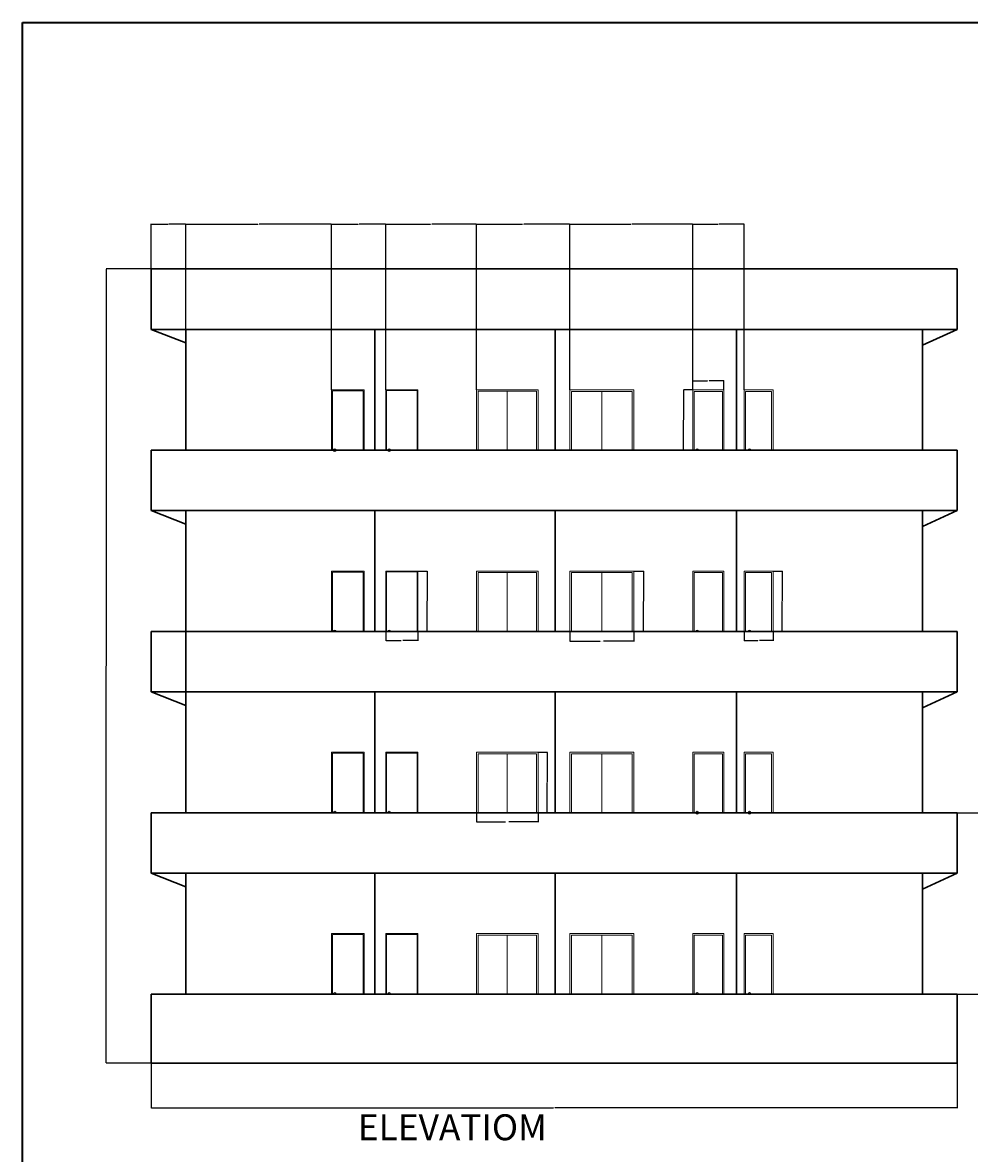
# Model space of a CAD drawing. Units: inches. Extents: x 1944 to 3454, y 1352 to 3055.
# Tile 16 of 17: x 1944 to 2602, y 2269 to 3055. Entities that reach past the tile are written whole.
import ezdxf

# ---------------------------------------------------------------- set-up
doc = ezdxf.new("R2010")
doc.units = ezdxf.units.IN
for name, color, linetype, lineweight in [('A-ANNO-DIMS', 2, 'Continuous', 18), ('A-ANNO-TITL', 7, 'Continuous', 30), ('A-ANNO-TTLB', 7, 'Continuous', 35), ('A-ELEV', 7, 'Continuous', 30), ('A-ELEV-DOOR', 3, 'Continuous', 18), ('A-ELEV-GLAZ', 4, 'Continuous', 18)]:
    doc.layers.add(name, color=color, linetype=linetype, lineweight=lineweight)
doc.styles.get("Standard").update_dxf_attribs({"font": 'arial.ttf'})
doc.dimstyles.get("Standard").update_dxf_attribs({"dimtxt": 0.18, "dimasz": 0.18, "dimexe": 0.18, "dimexo": 0.0625, "dimgap": 0.09, "dimtad": 0, "dimtih": 1, "dimtoh": 1, "dimdec": 4, "dimzin": 0, "dimdsep": 46, "dimtxsty": 'Standard', "dimcen": 0.09, "dimadec": 0, "dimazin": 0, "dimtfac": 1, "dimtdec": 4, "dimtofl": 0, "dimtmove": 0, "dimatfit": 3, "dimfxl": 1, "dimtolj": 1, "dimtzin": 0, "dimarcsym": 0})

# ---------------------------------------------------------------- blocks, each defined once
blk = doc.blocks.new('ELEV-DOOR-22.35IN-01')
for p, q in [((0, 42), (0, 0)), ((0, 42), (22.35, 42)), ((0, 42), (0, 0)), ((0, 42), (22.35, 42)), ((22.35, 42), (22.35, 0)), ((22.35, 42), (22.35, 0))]:
    blk.add_line(p, q)
blk.add_lwpolyline([(0.46, 0), (0.46, 41.46), (21.87, 41.46), (21.87, 0)])
blk.add_arc((2.34, 0), 0.993, 0, 180)
blk = doc.blocks.new('ELEV-DOOR-21.74IN-01')
for p, q in [((0, 42), (0, 0)), ((0, 42), (21.74, 42)), ((0, 42), (0, 0)), ((0, 42), (21.74, 42)), ((21.74, 42), (21.74, 0)), ((21.74, 42), (21.74, 0))]:
    blk.add_line(p, q)
blk.add_lwpolyline([(1.03, 0), (1.03, 40.92), (20.81, 40.92), (20.81, 0)])
blk.add_arc((3.12, 0), 0.993, 0, 180)
blk = doc.blocks.new('ELEV-DOOR-20.24IN-01')
for p, q in [((0, 42), (0, 0)), ((0, 42), (20.24, 42)), ((0, 42), (0, 0)), ((0, 42), (20.24, 42)), ((20.24, 42), (20.24, 0)), ((20.24, 42), (20.24, 0))]:
    blk.add_line(p, q)
blk.add_lwpolyline([(1.07, 0), (1.07, 40.9), (18.98, 40.9), (18.98, 0)])
blk.add_arc((3.81, 0), 0.993, 0, 180)
blk = doc.blocks.new('ELEV-GLAZ-42.86IN-01')
for p, q in [((0, 42), (0, 0)), ((0, 42), (42.86, 42)), ((0, 42), (0, 0)), ((0, 42), (42.86, 42)), ((21.49, 41), (21.49, 0)), ((42.86, 42), (42.86, 0)), ((42.86, 42), (42.86, 0))]:
    blk.add_line(p, q)
blk.add_lwpolyline([(1.15, 0), (1.15, 41), (41.83, 41), (41.83, 0)])
blk = doc.blocks.new('ELEV-GLAZ-44.51IN-01')
for p, q in [((0, 42), (0, 0)), ((0, 42), (44.51, 42)), ((0, 42), (0, 0)), ((0, 42), (44.51, 42)), ((22.21, 40.89), (22.21, 0)), ((44.51, 42), (44.51, 0)), ((44.51, 42), (44.51, 0))]:
    blk.add_line(p, q)
blk.add_lwpolyline([(1.11, 0), (1.11, 40.89), (43.32, 40.89), (43.32, 0)])
blk = doc.blocks.new('*D162')
at = {"layer": 'A-ANNO-DIMS', "color": 0, "lineweight": -2, "transparency": 16777216}
for p, q in [((2259.53, 2505.32), (2259.53, 2498.78)), ((2302.38, 2505.32), (2302.38, 2498.78)), ((2259.71, 2498.96), (2279.84, 2498.96)), ((2302.2, 2498.96), (2282.07, 2498.96))]:
    blk.add_line(p, q, dxfattribs=at)
at = {"layer": 'A-ANNO-DIMS', "color": 0, "transparency": 16777216}
for points in [[(2259.71, 2498.99), (2259.71, 2498.93), (2259.53, 2498.96)], [(2302.2, 2498.99), (2302.2, 2498.93), (2302.38, 2498.96)]]:
    blk.add_solid(points, dxfattribs=at)
at = {"layer": 'Defpoints', "color": 0, "transparency": 16777216}
for p in [(2259.53, 2505.38), (2302.38, 2505.38), (2302.38, 2498.96)]:
    blk.add_point(p, dxfattribs=at)
at = {"layer": 'A-ANNO-DIMS', "color": 0, "transparency": 16777216, "insert": (2280.96, 2498.96), "char_height": 0.18, "attachment_point": 5}
blk.add_mtext('\\A1;GLAZING 43 TYP.', dxfattribs=at)
blk = doc.blocks.new('*D163')
at = {"layer": 'A-ANNO-DIMS', "color": 0, "lineweight": -2, "transparency": 16777216}
for p, q in [((2302.45, 2547.38), (2308.99, 2547.38)), ((2308.81, 2547.2), (2308.81, 2526.56)), ((2308.81, 2505.56), (2308.81, 2526.2)), ((2302.45, 2505.38), (2308.99, 2505.38))]:
    blk.add_line(p, q, dxfattribs=at)
at = {"layer": 'A-ANNO-DIMS', "color": 0, "transparency": 16777216}
for points in [[(2308.78, 2547.2), (2308.84, 2547.2), (2308.81, 2547.38)], [(2308.78, 2505.56), (2308.84, 2505.56), (2308.81, 2505.38)]]:
    blk.add_solid(points, dxfattribs=at)
at = {"layer": 'Defpoints', "color": 0, "transparency": 16777216}
for p in [(2302.38, 2547.38), (2308.81, 2547.38), (2302.38, 2505.38)]:
    blk.add_point(p, dxfattribs=at)
at = {"layer": 'A-ANNO-DIMS', "color": 0, "transparency": 16777216, "insert": (2308.81, 2526.38), "char_height": 0.18, "attachment_point": 5}
blk.add_mtext('\\A1;42 TYP.', dxfattribs=at)
blk = doc.blocks.new('*D164')
at = {"layer": 'A-ANNO-DIMS', "color": 0, "lineweight": -2, "transparency": 16777216}
for p, q in [((2324.52, 2631.32), (2324.52, 2624.53)), ((2369.03, 2631.32), (2369.03, 2624.53)), ((2324.7, 2624.71), (2345.66, 2624.71)), ((2368.85, 2624.71), (2347.89, 2624.71))]:
    blk.add_line(p, q, dxfattribs=at)
at = {"layer": 'A-ANNO-DIMS', "color": 0, "transparency": 16777216}
for points in [[(2324.7, 2624.74), (2324.7, 2624.68), (2324.52, 2624.71)], [(2368.85, 2624.74), (2368.85, 2624.68), (2369.03, 2624.71)]]:
    blk.add_solid(points, dxfattribs=at)
at = {"layer": 'Defpoints', "color": 0, "transparency": 16777216}
for p in [(2324.52, 2631.38), (2369.03, 2631.38), (2369.03, 2624.71)]:
    blk.add_point(p, dxfattribs=at)
at = {"layer": 'A-ANNO-DIMS', "color": 0, "transparency": 16777216, "insert": (2346.78, 2624.71), "char_height": 0.18, "attachment_point": 5}
blk.add_mtext('\\A1;GLAZING 45 TYP.', dxfattribs=at)
blk = doc.blocks.new('*D165')
at = {"layer": 'A-ANNO-DIMS', "color": 0, "lineweight": -2, "transparency": 16777216}
for p, q in [((2369.1, 2673.38), (2375.89, 2673.38)), ((2375.71, 2673.2), (2375.71, 2652.56)), ((2375.71, 2631.56), (2375.71, 2652.2)), ((2369.1, 2631.38), (2375.89, 2631.38))]:
    blk.add_line(p, q, dxfattribs=at)
at = {"layer": 'A-ANNO-DIMS', "color": 0, "transparency": 16777216}
for points in [[(2375.68, 2673.2), (2375.74, 2673.2), (2375.71, 2673.38)], [(2375.68, 2631.56), (2375.74, 2631.56), (2375.71, 2631.38)]]:
    blk.add_solid(points, dxfattribs=at)
at = {"layer": 'Defpoints', "color": 0, "transparency": 16777216}
for p in [(2369.03, 2673.38), (2375.71, 2673.38), (2369.03, 2631.38)]:
    blk.add_point(p, dxfattribs=at)
at = {"layer": 'A-ANNO-DIMS', "color": 0, "transparency": 16777216, "insert": (2375.71, 2652.38), "char_height": 0.18, "attachment_point": 5}
blk.add_mtext('\\A1;42 TYP.', dxfattribs=at)
blk = doc.blocks.new('*D166')
at = {"layer": 'A-ANNO-DIMS', "color": 0, "lineweight": -2, "transparency": 16777216}
for p, q in [((2218.95, 2673.38), (2225.37, 2673.38)), ((2225.19, 2673.2), (2225.19, 2652.57)), ((2225.19, 2631.56), (2225.19, 2652.2)), ((2218.95, 2631.38), (2225.37, 2631.38))]:
    blk.add_line(p, q, dxfattribs=at)
at = {"layer": 'A-ANNO-DIMS', "color": 0, "transparency": 16777216}
for points in [[(2225.16, 2673.2), (2225.22, 2673.2), (2225.19, 2673.38)], [(2225.16, 2631.56), (2225.22, 2631.56), (2225.19, 2631.38)]]:
    blk.add_solid(points, dxfattribs=at)
at = {"layer": 'Defpoints', "color": 0, "transparency": 16777216}
for p in [(2218.89, 2673.38), (2225.19, 2673.38), (2218.89, 2631.38)]:
    blk.add_point(p, dxfattribs=at)
at = {"layer": 'A-ANNO-DIMS', "color": 0, "transparency": 16777216, "insert": (2225.19, 2652.38), "char_height": 0.18, "attachment_point": 5}
blk.add_mtext('\\A1;DOOR 42 TYP.', dxfattribs=at)
blk = doc.blocks.new('*D167')
at = {"layer": 'A-ANNO-DIMS', "color": 0, "lineweight": -2, "transparency": 16777216}
for p, q in [((2196.54, 2631.32), (2196.54, 2624.9)), ((2218.89, 2631.32), (2218.89, 2624.9)), ((2196.72, 2625.08), (2207.18, 2625.08)), ((2218.71, 2625.08), (2208.24, 2625.08))]:
    blk.add_line(p, q, dxfattribs=at)
at = {"layer": 'A-ANNO-DIMS', "color": 0, "transparency": 16777216}
for points in [[(2196.72, 2625.11), (2196.72, 2625.05), (2196.54, 2625.08)], [(2218.71, 2625.11), (2218.71, 2625.05), (2218.89, 2625.08)]]:
    blk.add_solid(points, dxfattribs=at)
at = {"layer": 'Defpoints', "color": 0, "transparency": 16777216}
for p in [(2196.54, 2631.38), (2218.89, 2631.38), (2218.89, 2625.08)]:
    blk.add_point(p, dxfattribs=at)
at = {"layer": 'A-ANNO-DIMS', "color": 0, "transparency": 16777216, "insert": (2207.71, 2625.08), "char_height": 0.18, "attachment_point": 5}
blk.add_mtext('\\A1;22 TYP.', dxfattribs=at)
blk = doc.blocks.new('*D168')
at = {"layer": 'A-ANNO-DIMS', "color": 0, "lineweight": -2, "transparency": 16777216}
for p, q in [((2409.85, 2799.38), (2403.43, 2799.38)), ((2403.61, 2799.2), (2403.61, 2778.57)), ((2403.61, 2757.56), (2403.61, 2778.2)), ((2409.85, 2757.38), (2403.43, 2757.38))]:
    blk.add_line(p, q, dxfattribs=at)
at = {"layer": 'A-ANNO-DIMS', "color": 0, "transparency": 16777216}
for points in [[(2403.58, 2799.2), (2403.64, 2799.2), (2403.61, 2799.38)], [(2403.58, 2757.56), (2403.64, 2757.56), (2403.61, 2757.38)]]:
    blk.add_solid(points, dxfattribs=at)
at = {"layer": 'Defpoints', "color": 0, "transparency": 16777216}
for p in [(2403.61, 2799.38), (2409.91, 2799.38), (2409.91, 2757.38)]:
    blk.add_point(p, dxfattribs=at)
at = {"layer": 'A-ANNO-DIMS', "color": 0, "transparency": 16777216, "insert": (2403.61, 2778.38), "char_height": 0.18, "attachment_point": 5}
blk.add_mtext('\\A1;DOOR 42 TYP.', dxfattribs=at)
blk = doc.blocks.new('*D169')
at = {"layer": 'A-ANNO-DIMS', "color": 0, "lineweight": -2, "transparency": 16777216}
for p, q in [((2409.91, 2799.45), (2409.91, 2805.86)), ((2410.09, 2805.68), (2420.26, 2805.68)), ((2431.48, 2805.68), (2421.31, 2805.68)), ((2431.66, 2799.45), (2431.66, 2805.86))]:
    blk.add_line(p, q, dxfattribs=at)
at = {"layer": 'A-ANNO-DIMS', "color": 0, "transparency": 16777216}
for points in [[(2410.09, 2805.71), (2410.09, 2805.65), (2409.91, 2805.68)], [(2431.48, 2805.71), (2431.48, 2805.65), (2431.66, 2805.68)]]:
    blk.add_solid(points, dxfattribs=at)
at = {"layer": 'Defpoints', "color": 0, "transparency": 16777216}
for p in [(2409.91, 2799.38), (2431.66, 2805.68), (2431.66, 2799.38)]:
    blk.add_point(p, dxfattribs=at)
at = {"layer": 'A-ANNO-DIMS', "color": 0, "transparency": 16777216, "insert": (2420.79, 2805.68), "char_height": 0.18, "attachment_point": 5}
blk.add_mtext('\\A1;22 TYP.', dxfattribs=at)
blk = doc.blocks.new('*D170')
at = {"layer": 'A-ANNO-DIMS', "color": 0, "lineweight": -2, "transparency": 16777216}
for p, q in [((2465.95, 2673.38), (2472.37, 2673.38)), ((2472.19, 2673.2), (2472.19, 2652.57)), ((2472.19, 2631.56), (2472.19, 2652.2)), ((2465.95, 2631.38), (2472.37, 2631.38))]:
    blk.add_line(p, q, dxfattribs=at)
at = {"layer": 'A-ANNO-DIMS', "color": 0, "transparency": 16777216}
for points in [[(2472.16, 2673.2), (2472.22, 2673.2), (2472.19, 2673.38)], [(2472.16, 2631.56), (2472.22, 2631.56), (2472.19, 2631.38)]]:
    blk.add_solid(points, dxfattribs=at)
at = {"layer": 'Defpoints', "color": 0, "transparency": 16777216}
for p in [(2465.89, 2673.38), (2472.19, 2673.38), (2465.89, 2631.38)]:
    blk.add_point(p, dxfattribs=at)
at = {"layer": 'A-ANNO-DIMS', "color": 0, "transparency": 16777216, "insert": (2472.19, 2652.38), "char_height": 0.18, "attachment_point": 5}
blk.add_mtext('\\A1;DOOR 42 TYP.', dxfattribs=at)
blk = doc.blocks.new('*D171')
at = {"layer": 'A-ANNO-DIMS', "color": 0, "lineweight": -2, "transparency": 16777216}
for p, q in [((2445.66, 2631.32), (2445.66, 2624.9)), ((2465.89, 2631.32), (2465.89, 2624.9)), ((2445.84, 2625.08), (2455.24, 2625.08)), ((2465.71, 2625.08), (2456.3, 2625.08))]:
    blk.add_line(p, q, dxfattribs=at)
at = {"layer": 'A-ANNO-DIMS', "color": 0, "transparency": 16777216}
for points in [[(2445.84, 2625.11), (2445.84, 2625.05), (2445.66, 2625.08)], [(2465.71, 2625.11), (2465.71, 2625.05), (2465.89, 2625.08)]]:
    blk.add_solid(points, dxfattribs=at)
at = {"layer": 'Defpoints', "color": 0, "transparency": 16777216}
for p in [(2445.66, 2631.38), (2465.89, 2631.38), (2465.89, 2625.08)]:
    blk.add_point(p, dxfattribs=at)
at = {"layer": 'A-ANNO-DIMS', "color": 0, "transparency": 16777216, "insert": (2455.77, 2625.08), "char_height": 0.18, "attachment_point": 5}
blk.add_mtext('\\A1;20 TYP.', dxfattribs=at)
blk = doc.blocks.new('*D199')
at = {"layer": 'A-ANNO-DIMS', "color": 0, "lineweight": -2, "transparency": 16777216}
for p, q in [((2033.32, 2331.32), (2033.32, 2300)), ((2593.82, 2331.32), (2593.82, 2300)), ((2033.5, 2300.18), (2313.18, 2300.18)), ((2593.64, 2300.18), (2313.97, 2300.18))]:
    blk.add_line(p, q, dxfattribs=at)
at = {"layer": 'A-ANNO-DIMS', "color": 0, "transparency": 16777216}
for points in [[(2033.5, 2300.21), (2033.5, 2300.15), (2033.32, 2300.18)], [(2593.64, 2300.21), (2593.64, 2300.15), (2593.82, 2300.18)]]:
    blk.add_solid(points, dxfattribs=at)
at = {"layer": 'Defpoints', "color": 0, "transparency": 16777216}
for p in [(2033.32, 2331.38), (2593.82, 2331.38), (2593.82, 2300.18)]:
    blk.add_point(p, dxfattribs=at)
at = {"layer": 'A-ANNO-DIMS', "color": 0, "transparency": 16777216, "insert": (2313.57, 2300.18), "char_height": 0.18, "attachment_point": 5}
blk.add_mtext('\\A1;560.5', dxfattribs=at)
blk = doc.blocks.new('*D200')
at = {"layer": 'A-ANNO-DIMS', "color": 0, "lineweight": -2, "transparency": 16777216}
for p, q in [((2033.26, 2883.38), (2001.94, 2883.38)), ((2002.12, 2883.2), (2002.12, 2607.57)), ((2002.12, 2331.56), (2002.12, 2607.2)), ((2033.26, 2331.38), (2001.94, 2331.38))]:
    blk.add_line(p, q, dxfattribs=at)
at = {"layer": 'A-ANNO-DIMS', "color": 0, "transparency": 16777216}
for points in [[(2002.09, 2883.2), (2002.15, 2883.2), (2002.12, 2883.38)], [(2002.09, 2331.56), (2002.15, 2331.56), (2002.12, 2331.38)]]:
    blk.add_solid(points, dxfattribs=at)
at = {"layer": 'Defpoints', "color": 0, "transparency": 16777216}
for p in [(2002.12, 2883.38), (2033.32, 2883.38), (2033.32, 2331.38)]:
    blk.add_point(p, dxfattribs=at)
at = {"layer": 'A-ANNO-DIMS', "color": 0, "transparency": 16777216, "insert": (2002.12, 2607.38), "char_height": 0.18, "attachment_point": 5}
blk.add_mtext('\\A1;552', dxfattribs=at)
blk = doc.blocks.new('*D201')
at = {"layer": 'A-ANNO-DIMS', "color": 0, "lineweight": -2, "transparency": 16777216}
for p, q in [((2593.88, 2505.38), (2625.2, 2505.38)), ((2625.02, 2505.2), (2625.02, 2442.57)), ((2625.02, 2379.56), (2625.02, 2442.2)), ((2593.88, 2379.38), (2625.2, 2379.38))]:
    blk.add_line(p, q, dxfattribs=at)
at = {"layer": 'A-ANNO-DIMS', "color": 0, "transparency": 16777216}
for points in [[(2624.99, 2505.2), (2625.05, 2505.2), (2625.02, 2505.38)], [(2624.99, 2379.56), (2625.05, 2379.56), (2625.02, 2379.38)]]:
    blk.add_solid(points, dxfattribs=at)
at = {"layer": 'Defpoints', "color": 0, "transparency": 16777216}
for p in [(2593.82, 2505.38), (2625.02, 2505.38), (2593.82, 2379.38)]:
    blk.add_point(p, dxfattribs=at)
at = {"layer": 'A-ANNO-DIMS', "color": 0, "transparency": 16777216, "insert": (2625.02, 2442.38), "char_height": 0.18, "attachment_point": 5}
blk.add_mtext('\\A1;126', dxfattribs=at)
blk = doc.blocks.new('*D202')
at = {"layer": 'A-ANNO-DIMS', "color": 0, "lineweight": -2, "transparency": 16777216}
for p, q in [((2033.32, 2841.45), (2033.32, 2914.76)), ((2033.5, 2914.58), (2045.1, 2914.58)), ((2057.14, 2914.58), (2045.54, 2914.58)), ((2057.32, 2841.45), (2057.32, 2914.76))]:
    blk.add_line(p, q, dxfattribs=at)
at = {"layer": 'A-ANNO-DIMS', "color": 0, "transparency": 16777216}
for points in [[(2033.5, 2914.61), (2033.5, 2914.55), (2033.32, 2914.58)], [(2057.14, 2914.61), (2057.14, 2914.55), (2057.32, 2914.58)]]:
    blk.add_solid(points, dxfattribs=at)
at = {"layer": 'Defpoints', "color": 0, "transparency": 16777216}
for p in [(2057.32, 2914.58), (2033.32, 2841.38), (2057.32, 2841.38)]:
    blk.add_point(p, dxfattribs=at)
at = {"layer": 'A-ANNO-DIMS', "color": 0, "transparency": 16777216, "insert": (2045.32, 2914.58), "char_height": 0.18, "attachment_point": 5}
blk.add_mtext('\\A1;24', dxfattribs=at)
blk = doc.blocks.new('*D203')
at = {"layer": 'A-ANNO-DIMS', "color": 0, "lineweight": -2, "transparency": 16777216}
for p, q in [((2057.32, 2841.45), (2057.32, 2914.76)), ((2057.5, 2914.58), (2107.56, 2914.58)), ((2158.52, 2914.58), (2108.47, 2914.58)), ((2158.7, 2799.45), (2158.7, 2914.76))]:
    blk.add_line(p, q, dxfattribs=at)
at = {"layer": 'A-ANNO-DIMS', "color": 0, "transparency": 16777216}
for points in [[(2057.5, 2914.61), (2057.5, 2914.55), (2057.32, 2914.58)], [(2158.52, 2914.61), (2158.52, 2914.55), (2158.7, 2914.58)]]:
    blk.add_solid(points, dxfattribs=at)
at = {"layer": 'Defpoints', "color": 0, "transparency": 16777216}
for p in [(2158.7, 2914.58), (2057.32, 2841.38), (2158.7, 2799.38)]:
    blk.add_point(p, dxfattribs=at)
at = {"layer": 'A-ANNO-DIMS', "color": 0, "transparency": 16777216, "insert": (2108.01, 2914.58), "char_height": 0.18, "attachment_point": 5}
blk.add_mtext('\\A1;101.38', dxfattribs=at)
blk = doc.blocks.new('*D204')
at = {"layer": 'A-ANNO-DIMS', "color": 0, "lineweight": -2, "transparency": 16777216}
for p, q in [((2158.7, 2799.45), (2158.7, 2914.76)), ((2158.88, 2914.58), (2177.23, 2914.58)), ((2196.36, 2914.58), (2178.01, 2914.58)), ((2196.54, 2799.45), (2196.54, 2914.76))]:
    blk.add_line(p, q, dxfattribs=at)
at = {"layer": 'A-ANNO-DIMS', "color": 0, "transparency": 16777216}
for points in [[(2158.88, 2914.61), (2158.88, 2914.55), (2158.7, 2914.58)], [(2196.36, 2914.61), (2196.36, 2914.55), (2196.54, 2914.58)]]:
    blk.add_solid(points, dxfattribs=at)
at = {"layer": 'Defpoints', "color": 0, "transparency": 16777216}
for p in [(2196.54, 2914.58), (2158.7, 2799.38), (2196.54, 2799.38)]:
    blk.add_point(p, dxfattribs=at)
at = {"layer": 'A-ANNO-DIMS', "color": 0, "transparency": 16777216, "insert": (2177.62, 2914.58), "char_height": 0.18, "attachment_point": 5}
blk.add_mtext('\\A1;37.84', dxfattribs=at)
blk = doc.blocks.new('*D205')
at = {"layer": 'A-ANNO-DIMS', "color": 0, "lineweight": -2, "transparency": 16777216}
for p, q in [((2196.54, 2799.45), (2196.54, 2914.76)), ((2196.72, 2914.58), (2227.64, 2914.58)), ((2259.35, 2914.58), (2228.43, 2914.58)), ((2259.53, 2799.45), (2259.53, 2914.76))]:
    blk.add_line(p, q, dxfattribs=at)
at = {"layer": 'A-ANNO-DIMS', "color": 0, "transparency": 16777216}
for points in [[(2196.72, 2914.61), (2196.72, 2914.55), (2196.54, 2914.58)], [(2259.35, 2914.61), (2259.35, 2914.55), (2259.53, 2914.58)]]:
    blk.add_solid(points, dxfattribs=at)
at = {"layer": 'Defpoints', "color": 0, "transparency": 16777216}
for p in [(2259.53, 2914.58), (2196.54, 2799.38), (2259.53, 2799.38)]:
    blk.add_point(p, dxfattribs=at)
at = {"layer": 'A-ANNO-DIMS', "color": 0, "transparency": 16777216, "insert": (2228.03, 2914.58), "char_height": 0.18, "attachment_point": 5}
blk.add_mtext('\\A1;62.99', dxfattribs=at)
blk = doc.blocks.new('*D206')
at = {"layer": 'A-ANNO-DIMS', "color": 0, "lineweight": -2, "transparency": 16777216}
for p, q in [((2259.53, 2799.45), (2259.53, 2914.76)), ((2259.71, 2914.58), (2291.63, 2914.58)), ((2324.34, 2914.58), (2292.42, 2914.58)), ((2324.52, 2799.45), (2324.52, 2914.76))]:
    blk.add_line(p, q, dxfattribs=at)
at = {"layer": 'A-ANNO-DIMS', "color": 0, "transparency": 16777216}
for points in [[(2259.71, 2914.61), (2259.71, 2914.55), (2259.53, 2914.58)], [(2324.34, 2914.61), (2324.34, 2914.55), (2324.52, 2914.58)]]:
    blk.add_solid(points, dxfattribs=at)
at = {"layer": 'Defpoints', "color": 0, "transparency": 16777216}
for p in [(2324.52, 2914.58), (2259.53, 2799.38), (2324.52, 2799.38)]:
    blk.add_point(p, dxfattribs=at)
at = {"layer": 'A-ANNO-DIMS', "color": 0, "transparency": 16777216, "insert": (2292.03, 2914.58), "char_height": 0.18, "attachment_point": 5}
blk.add_mtext('\\A1;64.99', dxfattribs=at)
blk = doc.blocks.new('*D207')
at = {"layer": 'A-ANNO-DIMS', "color": 0, "lineweight": -2, "transparency": 16777216}
for p, q in [((2324.52, 2799.45), (2324.52, 2914.76)), ((2324.7, 2914.58), (2366.89, 2914.58)), ((2409.73, 2914.58), (2367.54, 2914.58)), ((2409.91, 2799.45), (2409.91, 2914.76))]:
    blk.add_line(p, q, dxfattribs=at)
at = {"layer": 'A-ANNO-DIMS', "color": 0, "transparency": 16777216}
for points in [[(2324.7, 2914.61), (2324.7, 2914.55), (2324.52, 2914.58)], [(2409.73, 2914.61), (2409.73, 2914.55), (2409.91, 2914.58)]]:
    blk.add_solid(points, dxfattribs=at)
at = {"layer": 'Defpoints', "color": 0, "transparency": 16777216}
for p in [(2409.91, 2914.58), (2324.52, 2799.38), (2409.91, 2799.38)]:
    blk.add_point(p, dxfattribs=at)
at = {"layer": 'A-ANNO-DIMS', "color": 0, "transparency": 16777216, "insert": (2367.22, 2914.58), "char_height": 0.18, "attachment_point": 5}
blk.add_mtext('\\A1;85.4', dxfattribs=at)
blk = doc.blocks.new('*D208')
at = {"layer": 'A-ANNO-DIMS', "color": 0, "lineweight": -2, "transparency": 16777216}
for p, q in [((2409.91, 2799.45), (2409.91, 2914.76)), ((2410.09, 2914.58), (2427.39, 2914.58)), ((2445.48, 2914.58), (2428.18, 2914.58)), ((2445.66, 2799.45), (2445.66, 2914.76))]:
    blk.add_line(p, q, dxfattribs=at)
at = {"layer": 'A-ANNO-DIMS', "color": 0, "transparency": 16777216}
for points in [[(2410.09, 2914.61), (2410.09, 2914.55), (2409.91, 2914.58)], [(2445.48, 2914.61), (2445.48, 2914.55), (2445.66, 2914.58)]]:
    blk.add_solid(points, dxfattribs=at)
at = {"layer": 'Defpoints', "color": 0, "transparency": 16777216}
for p in [(2445.66, 2914.58), (2409.91, 2799.38), (2445.66, 2799.38)]:
    blk.add_point(p, dxfattribs=at)
at = {"layer": 'A-ANNO-DIMS', "color": 0, "transparency": 16777216, "insert": (2427.78, 2914.58), "char_height": 0.18, "attachment_point": 5}
blk.add_mtext('\\A1;35.74', dxfattribs=at)

msp = doc.modelspace()

# ---------------------------------------------------------------- linework, layer by layer
at = {"layer": 'A-ANNO-TTLB'}
msp.add_lwpolyline([(1943.914, 3054.605), (3453.633, 3054.605), (3453.633, 1351.76), (1943.914, 1351.76)], close=True, dxfattribs=at)
at = {"layer": 'A-ELEV'}
for p, q in [((2033.322, 2883.384), (2593.822, 2883.384)), ((2033.322, 2841.384), (2033.322, 2883.384)), ((2593.822, 2841.384), (2593.822, 2883.384)), ((2033.322, 2841.384), (2593.822, 2841.384)), ((2033.322, 2841.384), (2057.322, 2831.986)), ((2057.322, 2841.384), (2057.322, 2757.384)), ((2188.947, 2757.384), (2188.947, 2841.384)), ((2314.352, 2757.384), (2314.352, 2841.384)), ((2440.322, 2757.384), (2440.322, 2841.384)), ((2569.822, 2841.384), (2569.822, 2757.384)), ((2593.822, 2841.384), (2569.822, 2830.307)), ((2033.322, 2757.384), (2593.822, 2757.384)), ((2033.322, 2715.384), (2033.322, 2757.384)), ((2593.822, 2715.384), (2593.822, 2757.384)), ((2033.322, 2715.384), (2593.822, 2715.384)), ((2033.322, 2715.384), (2057.322, 2705.986)), ((2057.322, 2715.384), (2057.322, 2583.384)), ((2057.322, 2715.384), (2057.322, 2709.384)), ((2188.947, 2631.384), (2188.947, 2715.384)), ((2314.352, 2631.384), (2314.352, 2715.384)), ((2440.322, 2631.384), (2440.322, 2715.384)), ((2569.822, 2715.384), (2569.822, 2631.384)), ((2569.822, 2715.384), (2569.822, 2709.384)), ((2593.822, 2715.384), (2569.822, 2704.307)), ((2033.322, 2631.384), (2593.822, 2631.384)), ((2033.322, 2589.384), (2033.322, 2631.384)), ((2057.322, 2631.384), (2057.322, 2505.384)), ((2593.822, 2589.384), (2593.822, 2631.384)), ((2033.322, 2589.384), (2593.822, 2589.384)), ((2033.322, 2589.384), (2057.322, 2579.986)), ((2188.947, 2505.384), (2188.947, 2589.384)), ((2314.352, 2505.384), (2314.352, 2589.384)), ((2440.322, 2505.384), (2440.322, 2589.384)), ((2569.822, 2589.384), (2569.822, 2505.384)), ((2569.822, 2589.384), (2569.822, 2583.384)), ((2593.822, 2589.384), (2569.822, 2578.307)), ((2033.322, 2505.384), (2593.822, 2505.384)), ((2033.322, 2463.384), (2033.322, 2505.384)), ((2593.822, 2463.384), (2593.822, 2505.384)), ((2033.322, 2463.384), (2593.822, 2463.384)), ((2033.322, 2463.384), (2057.322, 2453.986)), ((2057.322, 2463.384), (2057.322, 2379.384)), ((2057.322, 2463.384), (2057.322, 2457.384)), ((2188.947, 2379.384), (2188.947, 2463.384)), ((2314.352, 2379.384), (2314.352, 2463.384)), ((2440.322, 2379.384), (2440.322, 2463.384)), ((2569.822, 2463.384), (2569.822, 2379.384)), ((2569.822, 2463.384), (2569.822, 2457.384)), ((2593.822, 2463.384), (2569.822, 2452.307)), ((2033.322, 2379.384), (2593.822, 2379.384)), ((2033.322, 2331.384), (2033.322, 2379.384)), ((2593.822, 2331.384), (2593.822, 2379.384)), ((2057.322, 2331.384), (2033.322, 2331.384)), ((2057.322, 2331.384), (2569.822, 2331.384)), ((2569.822, 2331.384), (2593.822, 2331.384))]:
    msp.add_line(p, q, dxfattribs=at)
at = {"layer": 'A-ELEV-DOOR'}
for p, q in [((2158.703, 2799.384), (2158.703, 2757.384)), ((2158.703, 2799.384), (2181.354, 2799.384)), ((2158.703, 2799.384), (2158.703, 2757.384)), ((2158.703, 2799.384), (2181.354, 2799.384)), ((2181.354, 2799.384), (2181.354, 2757.384)), ((2181.354, 2799.384), (2181.354, 2757.384)), ((2196.54, 2799.384), (2196.54, 2757.384)), ((2196.54, 2799.384), (2218.889, 2799.384)), ((2196.54, 2799.384), (2196.54, 2757.384)), ((2196.54, 2799.384), (2218.889, 2799.384)), ((2218.889, 2799.384), (2218.889, 2757.384)), ((2218.889, 2799.384), (2218.889, 2757.384)), ((2158.703, 2673.384), (2158.703, 2631.384)), ((2158.703, 2673.384), (2181.354, 2673.384)), ((2158.703, 2673.384), (2158.703, 2631.384)), ((2158.703, 2673.384), (2181.354, 2673.384)), ((2181.354, 2673.384), (2181.354, 2631.384)), ((2181.354, 2673.384), (2181.354, 2631.384)), ((2158.703, 2547.384), (2158.703, 2505.384)), ((2158.703, 2547.384), (2181.354, 2547.384)), ((2158.703, 2547.384), (2158.703, 2505.384)), ((2158.703, 2547.384), (2181.354, 2547.384)), ((2181.354, 2547.384), (2181.354, 2505.384)), ((2181.354, 2547.384), (2181.354, 2505.384)), ((2409.913, 2547.384), (2409.913, 2505.384)), ((2409.913, 2547.384), (2431.658, 2547.384)), ((2409.913, 2547.384), (2409.913, 2505.384)), ((2409.913, 2547.384), (2431.658, 2547.384)), ((2431.658, 2547.384), (2431.658, 2505.384)), ((2431.658, 2547.384), (2431.658, 2505.384)), ((2445.656, 2547.384), (2445.656, 2505.384)), ((2445.656, 2547.384), (2465.892, 2547.384)), ((2445.656, 2547.384), (2445.656, 2505.384)), ((2445.656, 2547.384), (2465.892, 2547.384)), ((2465.892, 2547.384), (2465.892, 2505.384)), ((2465.892, 2547.384), (2465.892, 2505.384)), ((2158.703, 2421.384), (2158.703, 2379.384)), ((2158.703, 2421.384), (2181.354, 2421.384)), ((2181.354, 2421.384), (2181.354, 2379.384)), ((2196.54, 2421.384), (2196.54, 2379.384)), ((2196.54, 2421.384), (2218.889, 2421.384)), ((2218.889, 2421.384), (2218.889, 2379.384)), ((2409.913, 2421.384), (2409.913, 2379.384)), ((2409.913, 2421.384), (2431.658, 2421.384)), ((2431.658, 2421.384), (2431.658, 2379.384)), ((2445.656, 2421.384), (2445.656, 2379.384)), ((2445.656, 2421.384), (2465.892, 2421.384)), ((2465.892, 2421.384), (2465.892, 2379.384))]:
    msp.add_line(p, q, dxfattribs=at)
for points in [[(2159.331, 2757.384), (2159.331, 2798.71), (2180.868, 2798.71), (2180.868, 2757.384)], [(2197.004, 2757.384), (2197.004, 2798.842), (2218.411, 2798.842), (2218.411, 2757.384)], [(2159.331, 2631.384), (2159.331, 2672.71), (2180.868, 2672.71), (2180.868, 2631.384)], [(2159.331, 2505.384), (2159.331, 2546.71), (2180.868, 2546.71), (2180.868, 2505.384)], [(2410.943, 2505.384), (2410.943, 2546.307), (2430.724, 2546.307), (2430.724, 2505.384)], [(2446.731, 2505.384), (2446.731, 2546.283), (2464.64, 2546.283), (2464.64, 2505.384)], [(2159.331, 2379.384), (2159.331, 2420.71), (2180.868, 2420.71), (2180.868, 2379.384)], [(2197.004, 2379.384), (2197.004, 2420.842), (2218.411, 2420.842), (2218.411, 2379.384)], [(2410.943, 2379.384), (2410.943, 2420.307), (2430.724, 2420.307), (2430.724, 2379.384)], [(2446.731, 2379.384), (2446.731, 2420.283), (2464.64, 2420.283), (2464.64, 2379.384)]]:
    msp.add_lwpolyline(points, dxfattribs=at)
for centre in [(2160.946, 2757.384), (2198.877, 2757.384), (2413.034, 2505.384), (2449.466, 2505.384)]:
    msp.add_circle(centre, 0.993, dxfattribs=at)
for centre, start in [((2160.946, 2631.384), 360), ((2160.946, 2505.384), 0), ((2160.946, 2379.384), 0), ((2198.877, 2379.384), 0), ((2413.034, 2379.384), 0), ((2449.466, 2379.384), 0)]:
    msp.add_arc(centre, 0.993, start, 180, dxfattribs=at)
at = {"layer": 'A-ELEV-GLAZ'}
for p, q in [((2259.529, 2421.384), (2259.529, 2379.384)), ((2259.529, 2421.384), (2302.384, 2421.384)), ((2302.384, 2421.384), (2302.384, 2379.384)), ((2324.521, 2421.384), (2324.521, 2379.384)), ((2324.521, 2421.384), (2369.033, 2421.384)), ((2369.033, 2421.384), (2369.033, 2379.384)), ((2281.017, 2420.379), (2281.017, 2379.384)), ((2346.735, 2420.276), (2346.735, 2379.384))]:
    msp.add_line(p, q, dxfattribs=at)
for points in [[(2260.675, 2379.384), (2260.675, 2420.379), (2301.359, 2420.379), (2301.359, 2379.384)], [(2325.631, 2379.384), (2325.631, 2420.276), (2367.839, 2420.276), (2367.839, 2379.384)]]:
    msp.add_lwpolyline(points, dxfattribs=at)

# ---------------------------------------------------------------- block references
at = {"layer": 'A-ELEV-DOOR'}
for name, p in [('ELEV-DOOR-21.74IN-01', (2409.913, 2757.384)), ('ELEV-DOOR-20.24IN-01', (2445.656, 2757.384)), ('ELEV-DOOR-22.35IN-01', (2196.54, 2631.384)), ('ELEV-DOOR-21.74IN-01', (2409.913, 2631.384)), ('ELEV-DOOR-20.24IN-01', (2445.656, 2631.384)), ('ELEV-DOOR-22.35IN-01', (2196.54, 2505.384))]:
    msp.add_blockref(name, p, dxfattribs=at)
at = {"layer": 'A-ELEV-GLAZ'}
for name, p in [('ELEV-GLAZ-42.86IN-01', (2259.529, 2757.384)), ('ELEV-GLAZ-44.51IN-01', (2324.521, 2757.384)), ('ELEV-GLAZ-42.86IN-01', (2259.529, 2631.384)), ('ELEV-GLAZ-44.51IN-01', (2324.521, 2631.384)), ('ELEV-GLAZ-42.86IN-01', (2259.529, 2505.384)), ('ELEV-GLAZ-44.51IN-01', (2324.521, 2505.384))]:
    msp.add_blockref(name, p, dxfattribs=at)

# ---------------------------------------------------------------- texts
at = {"layer": 'A-ANNO-TITL', "insert": (2177.053, 2295.748), "char_height": 18, "attachment_point": 1}
msp.add_mtext_dynamic_manual_height_columns('ELEVATIOM', width=379.94986, gutter_width=12.5, heights=[0], dxfattribs=at)

# ---------------------------------------------------------------- dimensions: what is measured, and where the dimension line sits
at = {"layer": 'A-ANNO-DIMS'}
for base, p1, p2, override, picture, middle in [((2057.322, 2914.584), (2033.322, 2841.384), (2057.322, 2841.384), {"dimdec": 0, "dimlfac": 1, "dimrnd": 0, "dimzin": 0, "dimdsep": 46, "dimlunit": 2}, '*D202', (2045.322, 2914.584)), ((2158.703, 2914.584), (2057.322, 2841.384), (2158.703, 2799.384), {"dimdec": 2, "dimlfac": 1, "dimrnd": 0, "dimzin": 0, "dimdsep": 46, "dimlunit": 2}, '*D203', (2108.012, 2914.584)), ((2196.54, 2914.584), (2158.703, 2799.384), (2196.54, 2799.384), {"dimdec": 2, "dimlfac": 1, "dimrnd": 0, "dimzin": 0, "dimdsep": 46, "dimlunit": 2}, '*D204', (2177.621, 2914.584)), ((2259.529, 2914.584), (2196.54, 2799.384), (2259.529, 2799.384), {"dimdec": 2, "dimlfac": 1, "dimrnd": 0, "dimzin": 0, "dimdsep": 46, "dimlunit": 2}, '*D205', (2228.035, 2914.584)), ((2324.521, 2914.584), (2259.529, 2799.384), (2324.521, 2799.384), {"dimdec": 2, "dimlfac": 1, "dimrnd": 0, "dimzin": 0, "dimdsep": 46, "dimlunit": 2}, '*D206', (2292.025, 2914.584)), ((2409.913, 2914.584), (2324.521, 2799.384), (2409.913, 2799.384), {"dimdec": 1, "dimlfac": 1, "dimrnd": 0, "dimzin": 0, "dimdsep": 46, "dimlunit": 2}, '*D207', (2367.217, 2914.584)), ((2445.656, 2914.584), (2409.913, 2799.384), (2445.656, 2799.384), {"dimdec": 2, "dimlfac": 1, "dimrnd": 0, "dimzin": 0, "dimdsep": 46, "dimlunit": 2}, '*D208', (2427.785, 2914.584)), ((2593.822, 2300.184), (2033.322, 2331.384), (2593.822, 2331.384), {"dimdec": 1, "dimlfac": 1, "dimrnd": 0, "dimzin": 0, "dimdsep": 46, "dimlunit": 2}, '*D199', (2313.572, 2300.184))]:
    dim = msp.add_linear_dim(base=base, p1=p1, p2=p2, dimstyle='Standard', override=override, dxfattribs=at)
    dim.commit()
    dim.dimension.update_dxf_attribs({"geometry": picture, "text_midpoint": middle})
for base, p1, p2, picture, middle in [((2002.122, 2883.384), (2033.322, 2331.384), (2033.322, 2883.384), '*D200', (2002.122, 2607.384)), ((2625.022, 2505.384), (2593.822, 2379.384), (2593.822, 2505.384), '*D201', (2625.022, 2442.384))]:
    dim = msp.add_linear_dim(base=base, p1=p1, p2=p2, angle=90, dimstyle='Standard', override={"dimdec": 0, "dimlfac": 1, "dimrnd": 0, "dimzin": 0, "dimdsep": 46, "dimlunit": 2}, dxfattribs=at)
    dim.commit()
    dim.dimension.update_dxf_attribs({"geometry": picture, "text_midpoint": middle})
for base, p1, p2, text, picture, middle in [((2403.613, 2799.384), (2409.913, 2757.384), (2409.913, 2799.384), 'DOOR <> TYP.', '*D168', (2403.613, 2778.384)), ((2225.189, 2673.384), (2218.889, 2631.384), (2218.889, 2673.384), 'DOOR <> TYP.', '*D166', (2225.189, 2652.384)), ((2375.71, 2673.384), (2369.033, 2631.384), (2369.033, 2673.384), '<> TYP.', '*D165', (2375.71, 2652.384)), ((2472.192, 2673.384), (2465.892, 2631.384), (2465.892, 2673.384), 'DOOR <> TYP.', '*D170', (2472.192, 2652.384)), ((2308.813, 2547.384), (2302.384, 2505.384), (2302.384, 2547.384), '<> TYP.', '*D163', (2308.813, 2526.384))]:
    dim = msp.add_linear_dim(base=base, p1=p1, p2=p2, angle=90, text=text, dimstyle='Standard', override={"dimdec": 0, "dimlfac": 1, "dimrnd": 0, "dimzin": 0, "dimdsep": 46, "dimlunit": 2}, dxfattribs=at)
    dim.commit()
    dim.dimension.update_dxf_attribs({"geometry": picture, "text_midpoint": middle})
for base, p1, p2, text, picture, middle in [((2431.658, 2805.684), (2409.913, 2799.384), (2431.658, 2799.384), '<> TYP.', '*D169', (2420.785, 2805.684)), ((2218.889, 2625.084), (2196.54, 2631.384), (2218.889, 2631.384), '<> TYP.', '*D167', (2207.714, 2625.084)), ((2369.033, 2624.707), (2324.521, 2631.384), (2369.033, 2631.384), 'GLAZING <> TYP.', '*D164', (2346.777, 2624.707)), ((2465.892, 2625.084), (2445.656, 2631.384), (2465.892, 2631.384), '<> TYP.', '*D171', (2455.774, 2625.084)), ((2302.384, 2498.955), (2259.529, 2505.384), (2302.384, 2505.384), 'GLAZING <> TYP.', '*D162', (2280.957, 2498.955))]:
    dim = msp.add_linear_dim(base=base, p1=p1, p2=p2, text=text, dimstyle='Standard', override={"dimdec": 0, "dimlfac": 1, "dimrnd": 0, "dimzin": 0, "dimdsep": 46, "dimlunit": 2}, dxfattribs=at)
    dim.commit()
    dim.dimension.update_dxf_attribs({"geometry": picture, "text_midpoint": middle})

doc.saveas('drawing.dxf')
